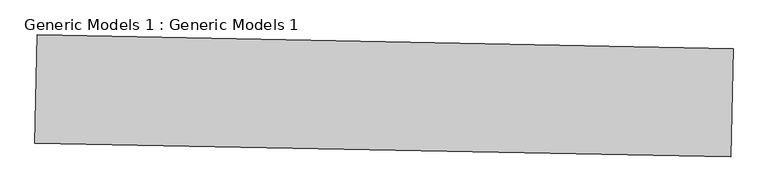
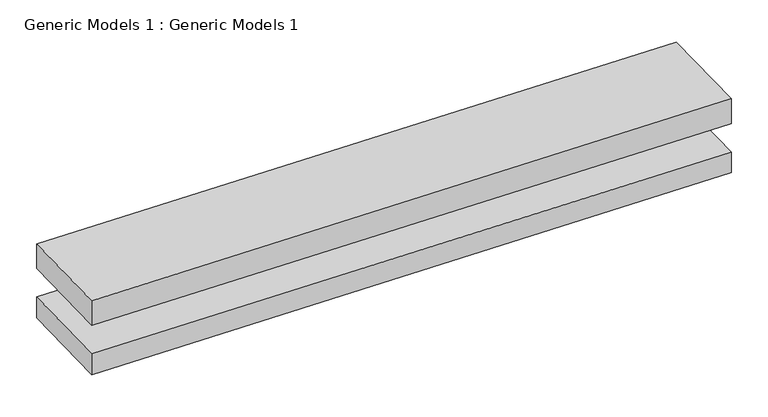
"""IFC4 building model written with IfcOpenShell, lengths in millimetres: proxy geometry, Generic Models 1 : Generic Models 1."""

from ifc_helpers import new_model, si_unit, frame, origin, place, context, project, spatial, polyline, outline, extrude, source, transform, mapped, element, save


def generic_models_1_generic_models_1_9ac678b9(model_context):
    return source(origin(), model_context, "Body", "SweptSolid", [
        extrude(outline(polyline([(-2755.4266589, -8862.7210526), (-8844.3060909, -8743.4809482), (-8825.7864312, -7797.7926202), (-2736.9069993, -7917.0327246), (-2755.4266589, -8862.7210526)])), frame((0.0, 0.0, 657.2987977), z_axis=(0.0, 0.0, 1.0), x_axis=(1.0, 0.0, 0.0)), (0.0, 0.0, 1.0), 250.3461462),
        extrude(outline(polyline([(-2755.4266589, -8862.7210526), (-8844.3060909, -8743.4809482), (-8825.7864312, -7797.7926202), (-2736.9069993, -7917.0327246), (-2755.4266589, -8862.7210526)])), frame((0.0, 0.0, 154.9867346), z_axis=(0.0, 0.0, 1.0), x_axis=(1.0, 0.0, 0.0)), (0.0, 0.0, 1.0), 211.539065),
    ])


if __name__ == "__main__":
    model = new_model("IFC4")
    model_context = context("Model", 3, world=origin())
    ifc_project = project(units=[si_unit("LENGTHUNIT", "METRE", prefix="MILLI")], contexts=[model_context])
    site = spatial("IfcSite", under=ifc_project)
    building = spatial("IfcBuilding", under=site)
    placement = place(None, origin())
    generic_models_1_generic_models_1_shape = generic_models_1_generic_models_1_9ac678b9(model_context)
    element("IfcBuildingElementProxy", 1, Name="Generic Models 1 : Generic Models 1", ObjectType="Generic Models 1 : Generic Models 1", at=placement, inside=building, context=model_context, shape_type="MappedRepresentation", body=[
        mapped(generic_models_1_generic_models_1_shape, transform((0.0, 0.0, 0.0), x_axis=(1.0, 0.0, 0.0), y_axis=(0.0, 1.0, 0.0), z_axis=(0.0, 0.0, 1.0))),
    ])
    save(model, "model.ifc")

# Revit data of these elements
# Element 1 (IfcBuildingElementProxy, "Generic Models 1 : Generic Models 1")
#   Materials on its faces: "Parking Stripe"
# Materials
#   "Parking Stripe": class "Paint", colour RGB 250 250 91, transparency 0, Cost = 0
